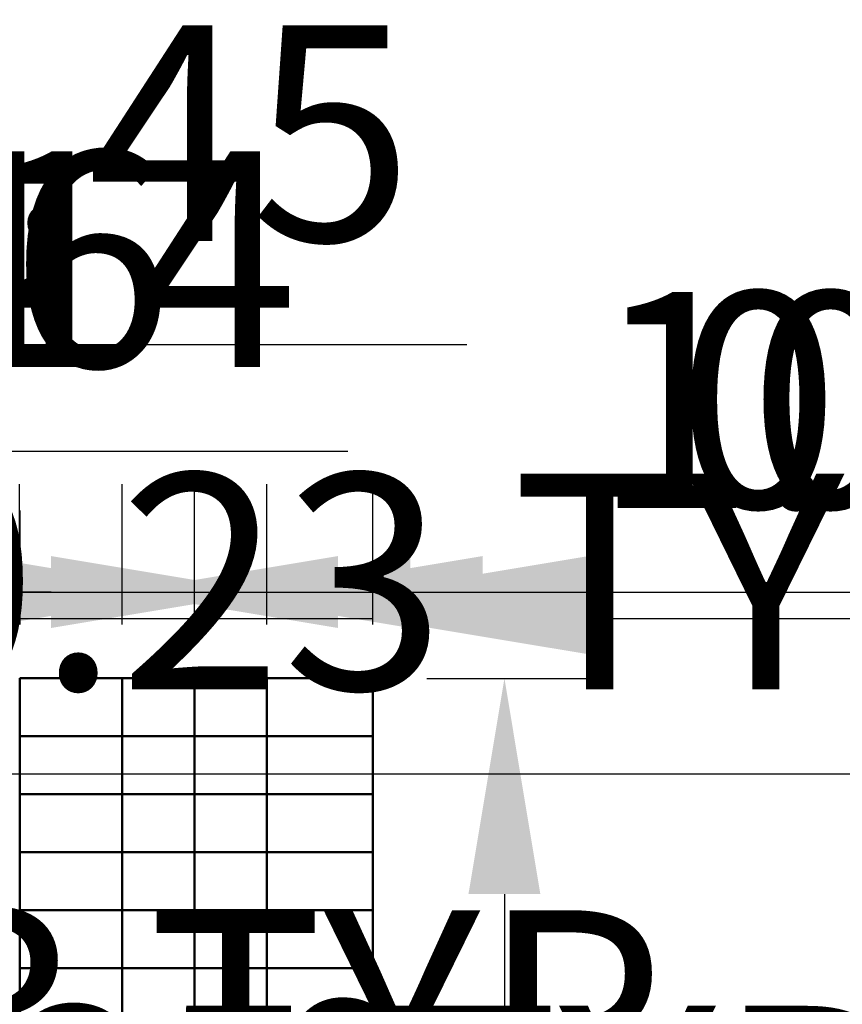
# Model space of a CAD drawing. Units: metres. Extents: x 782 to 1487, y 1262 to 7446.
# Tile 18 of 25: x 840.09 to 849.63, y 1302.06 to 1313.47. Entities that reach past the tile are written whole.
import ezdxf

# ---------------------------------------------------------------- set-up
doc = ezdxf.new("R2010")
doc.units = ezdxf.units.M
doc.layers.add('A-ANNO-DIMS', color=2, linetype='Continuous', lineweight=18)
doc.layers.add('A-WALL', color=7, linetype='Continuous', lineweight=50)
doc.styles.get("Standard").update_dxf_attribs({"font": 'arial.ttf'})
doc.dimstyles.new('ISO-25', dxfattribs={"dimtxt": 2.5, "dimasz": 2.5, "dimexe": 1.25, "dimexo": 0.625, "dimtad": 1, "dimtxsty": 'Standard', "dimcen": 2.5, "dimadec": 0, "dimazin": 0, "dimtfac": 1, "dimtmove": 0, "dimatfit": 3, "dimfxl": 1, "dimarcsym": 0})

# ---------------------------------------------------------------- blocks, each defined once
blk = doc.blocks.new('*D7')
at = {"layer": 'A-ANNO-DIMS', "color": 0, "lineweight": -2, "transparency": 16777216}
for p, q in [((827.962, 1307.952), (827.962, 1310.955)), ((832.412, 1307.952), (832.412, 1310.955)), ((825.462, 1309.705), (822.962, 1309.705)), ((827.962, 1309.705), (832.412, 1309.705)), ((834.912, 1309.705), (845.276, 1309.705))]:
    blk.add_line(p, q, dxfattribs=at)
at = {"layer": 'A-ANNO-DIMS', "color": 0, "transparency": 16777216}
for points in [[(825.462, 1310.122), (825.462, 1309.289), (827.962, 1309.705)], [(834.912, 1310.122), (834.912, 1309.289), (832.412, 1309.705)]]:
    blk.add_solid(points, dxfattribs=at)
at = {"layer": 'Defpoints', "color": 0, "transparency": 16777216}
for p in [(832.412, 1309.705), (827.962, 1307.327), (832.412, 1307.327)]:
    blk.add_point(p, dxfattribs=at)
at = {"layer": 'A-ANNO-DIMS', "color": 0, "transparency": 16777216, "insert": (841.344, 1311.828), "char_height": 2.5, "attachment_point": 5}
blk.add_mtext('4,45', dxfattribs=at)
blk = doc.blocks.new('*D8')
at = {"layer": 'A-ANNO-DIMS', "color": 0, "lineweight": -2, "transparency": 16777216}
for p, q in [((844.81, 1305.835), (846.96, 1305.835)), ((845.71, 1303.335), (845.71, 1292.805)), ((844.81, 1290.305), (846.96, 1290.305))]:
    blk.add_line(p, q, dxfattribs=at)
at = {"layer": 'A-ANNO-DIMS', "color": 0, "transparency": 16777216}
for points in [[(845.293, 1303.335), (846.126, 1303.335), (845.71, 1305.835)], [(845.293, 1292.805), (846.126, 1292.805), (845.71, 1290.305)]]:
    blk.add_solid(points, dxfattribs=at)
at = {"layer": 'Defpoints', "color": 0, "transparency": 16777216}
for p in [(844.185, 1305.835), (844.185, 1290.305), (845.71, 1290.305)]:
    blk.add_point(p, dxfattribs=at)
at = {"layer": 'A-ANNO-DIMS', "color": 0, "transparency": 16777216, "insert": (843.582, 1298.07), "char_height": 2.5, "attachment_point": 5, "rotation": 90}
blk.add_mtext('15,53', dxfattribs=at)
blk = doc.blocks.new('*D9')
at = {"layer": 'A-ANNO-DIMS', "color": 0, "lineweight": -2, "transparency": 16777216}
for p, q in [((840.095, 1306.46), (840.095, 1307.78)), ((844.185, 1306.46), (844.185, 1307.78)), ((837.595, 1306.53), (835.095, 1306.53)), ((840.095, 1306.53), (844.185, 1306.53)), ((846.685, 1306.53), (857.034, 1306.53))]:
    blk.add_line(p, q, dxfattribs=at)
at = {"layer": 'A-ANNO-DIMS', "color": 0, "transparency": 16777216}
for points in [[(837.595, 1306.947), (837.595, 1306.114), (840.095, 1306.53)], [(846.685, 1306.947), (846.685, 1306.114), (844.185, 1306.53)]]:
    blk.add_solid(points, dxfattribs=at)
at = {"layer": 'Defpoints', "color": 0, "transparency": 16777216}
for p in [(844.185, 1306.53), (840.095, 1305.835), (844.185, 1305.835)]:
    blk.add_point(p, dxfattribs=at)
at = {"layer": 'A-ANNO-DIMS', "color": 0, "transparency": 16777216, "insert": (853.11, 1308.658), "char_height": 2.5, "attachment_point": 5}
blk.add_mtext('4,09', dxfattribs=at)
blk = doc.blocks.new('*D21')
at = {"layer": 'A-ANNO-DIMS', "color": 0, "lineweight": -2, "transparency": 16777216}
for p, q in [((827.576, 1298.565), (825.076, 1298.565)), ((830.076, 1298.565), (830.923, 1298.565)), ((833.423, 1298.565), (852.255, 1298.565)), ((830.076, 1298.073), (830.076, 1297.315)), ((830.923, 1298.073), (830.923, 1297.315))]:
    blk.add_line(p, q, dxfattribs=at)
at = {"layer": 'A-ANNO-DIMS', "color": 0, "transparency": 16777216}
for points in [[(827.576, 1298.981), (827.576, 1298.148), (830.076, 1298.565)], [(833.423, 1298.981), (833.423, 1298.148), (830.923, 1298.565)]]:
    blk.add_solid(points, dxfattribs=at)
at = {"layer": 'Defpoints', "color": 0, "transparency": 16777216}
for p in [(830.076, 1298.698), (830.923, 1298.698), (830.923, 1298.565)]:
    blk.add_point(p, dxfattribs=at)
at = {"layer": 'A-ANNO-DIMS', "color": 0, "transparency": 16777216, "insert": (844.089, 1300.466), "char_height": 2.5, "attachment_point": 5}
blk.add_mtext('0.85 TYP.', dxfattribs=at)
blk = doc.blocks.new('*D24')
at = {"layer": 'A-ANNO-DIMS', "color": 0, "lineweight": -2, "transparency": 16777216}
for p, q in [((811.209, 1294.423), (808.709, 1294.423)), ((813.709, 1294.423), (814.559, 1294.423)), ((817.059, 1294.423), (852.649, 1294.423)), ((813.709, 1293.926), (813.709, 1293.173)), ((814.559, 1293.926), (814.559, 1293.173))]:
    blk.add_line(p, q, dxfattribs=at)
at = {"layer": 'A-ANNO-DIMS', "color": 0, "transparency": 16777216}
for points in [[(811.209, 1294.84), (811.209, 1294.006), (813.709, 1294.423)], [(817.059, 1294.84), (817.059, 1294.006), (814.559, 1294.423)]]:
    blk.add_solid(points, dxfattribs=at)
at = {"layer": 'Defpoints', "color": 0, "transparency": 16777216}
for p in [(813.709, 1294.551), (814.559, 1294.551), (814.559, 1294.423)]:
    blk.add_point(p, dxfattribs=at)
at = {"layer": 'A-ANNO-DIMS', "color": 0, "transparency": 16777216, "insert": (836.104, 1296.342), "char_height": 2.5, "attachment_point": 5}
blk.add_mtext('DOOR D2 0.85 TYP.', dxfattribs=at)
blk = doc.blocks.new('*D27')
at = {"layer": 'A-ANNO-DIMS', "color": 0, "lineweight": -2, "transparency": 16777216}
for p, q in [((825.463, 1299.672), (822.963, 1299.672)), ((827.963, 1299.672), (828.193, 1299.672)), ((830.693, 1299.672), (849.525, 1299.672)), ((827.963, 1299.184), (827.963, 1298.422)), ((828.193, 1299.184), (828.193, 1298.422))]:
    blk.add_line(p, q, dxfattribs=at)
at = {"layer": 'A-ANNO-DIMS', "color": 0, "transparency": 16777216}
for points in [[(825.463, 1300.088), (825.463, 1299.255), (827.963, 1299.672)], [(830.693, 1300.088), (830.693, 1299.255), (828.193, 1299.672)]]:
    blk.add_solid(points, dxfattribs=at)
at = {"layer": 'Defpoints', "color": 0, "transparency": 16777216}
for p in [(827.963, 1299.809), (828.193, 1299.809), (828.193, 1299.672)]:
    blk.add_point(p, dxfattribs=at)
at = {"layer": 'A-ANNO-DIMS', "color": 0, "transparency": 16777216, "insert": (841.359, 1301.574), "char_height": 2.5, "attachment_point": 5}
blk.add_mtext('0.23 TYP.', dxfattribs=at)
blk = doc.blocks.new('*D29')
at = {"layer": 'A-ANNO-DIMS', "color": 0, "lineweight": -2, "transparency": 16777216}
for p, q in [((829.683, 1304.73), (827.183, 1304.73)), ((832.183, 1304.73), (832.413, 1304.73)), ((834.913, 1304.73), (853.745, 1304.73)), ((832.183, 1304.242), (832.183, 1303.48)), ((832.413, 1304.242), (832.413, 1303.48))]:
    blk.add_line(p, q, dxfattribs=at)
at = {"layer": 'A-ANNO-DIMS', "color": 0, "transparency": 16777216}
for points in [[(829.683, 1305.146), (829.683, 1304.313), (832.183, 1304.73)], [(834.913, 1305.146), (834.913, 1304.313), (832.413, 1304.73)]]:
    blk.add_solid(points, dxfattribs=at)
at = {"layer": 'Defpoints', "color": 0, "transparency": 16777216}
for p in [(832.183, 1304.867), (832.413, 1304.867), (832.413, 1304.73)]:
    blk.add_point(p, dxfattribs=at)
at = {"layer": 'A-ANNO-DIMS', "color": 0, "transparency": 16777216, "insert": (845.579, 1306.632), "char_height": 2.5, "attachment_point": 5}
blk.add_mtext('0.23 TYP.', dxfattribs=at)
blk = doc.blocks.new('*D94')
at = {"layer": 'A-ANNO-DIMS', "color": 0, "lineweight": -2, "transparency": 16777216}
for p, q in [((827.962, 1307.952), (827.962, 1309.718)), ((828.406, 1307.953), (828.406, 1309.718)), ((825.462, 1308.468), (822.962, 1308.468)), ((827.962, 1308.468), (828.406, 1308.468)), ((830.906, 1308.468), (841.139, 1308.468))]:
    blk.add_line(p, q, dxfattribs=at)
at = {"layer": 'A-ANNO-DIMS', "color": 0, "transparency": 16777216}
for points in [[(825.462, 1308.884), (825.462, 1308.051), (827.962, 1308.468)], [(830.906, 1308.884), (830.906, 1308.051), (828.406, 1308.468)]]:
    blk.add_solid(points, dxfattribs=at)
at = {"layer": 'Defpoints', "color": 0, "transparency": 16777216}
for p in [(828.406, 1308.468), (827.962, 1307.327), (828.406, 1307.328)]:
    blk.add_point(p, dxfattribs=at)
at = {"layer": 'A-ANNO-DIMS', "color": 0, "transparency": 16777216, "insert": (837.273, 1310.369), "char_height": 2.5, "attachment_point": 5}
blk.add_mtext('0.44', dxfattribs=at)
blk = doc.blocks.new('*D95')
at = {"layer": 'A-ANNO-DIMS', "color": 0, "lineweight": -2, "transparency": 16777216}
for p, q in [((828.406, 1307.953), (828.406, 1309.718)), ((829.22, 1307.953), (829.22, 1309.718)), ((825.906, 1308.468), (823.406, 1308.468)), ((828.406, 1308.468), (829.22, 1308.468)), ((831.72, 1308.468), (843.896, 1308.468))]:
    blk.add_line(p, q, dxfattribs=at)
at = {"layer": 'A-ANNO-DIMS', "color": 0, "transparency": 16777216}
for points in [[(825.906, 1308.884), (825.906, 1308.051), (828.406, 1308.468)], [(831.72, 1308.884), (831.72, 1308.051), (829.22, 1308.468)]]:
    blk.add_solid(points, dxfattribs=at)
at = {"layer": 'Defpoints', "color": 0, "transparency": 16777216}
for p in [(829.22, 1308.468), (828.406, 1307.328), (829.22, 1307.328)]:
    blk.add_point(p, dxfattribs=at)
at = {"layer": 'A-ANNO-DIMS', "color": 0, "transparency": 16777216, "insert": (839.058, 1310.369), "char_height": 2.5, "attachment_point": 5}
blk.add_mtext('0.814', dxfattribs=at)
blk = doc.blocks.new('*D96')
at = {"layer": 'A-ANNO-DIMS', "color": 0, "lineweight": -2, "transparency": 16777216}
for p, q in [((829.22, 1307.953), (829.22, 1309.718)), ((829.682, 1307.722), (829.682, 1309.718)), ((826.72, 1308.468), (824.22, 1308.468)), ((829.22, 1308.468), (829.682, 1308.468)), ((832.182, 1308.468), (842.425, 1308.468))]:
    blk.add_line(p, q, dxfattribs=at)
at = {"layer": 'A-ANNO-DIMS', "color": 0, "transparency": 16777216}
for points in [[(826.72, 1308.884), (826.72, 1308.051), (829.22, 1308.468)], [(832.182, 1308.884), (832.182, 1308.051), (829.682, 1308.468)]]:
    blk.add_solid(points, dxfattribs=at)
at = {"layer": 'Defpoints', "color": 0, "transparency": 16777216}
for p in [(829.682, 1308.468), (829.22, 1307.328), (829.682, 1307.097)]:
    blk.add_point(p, dxfattribs=at)
at = {"layer": 'A-ANNO-DIMS', "color": 0, "transparency": 16777216, "insert": (838.554, 1310.369), "char_height": 2.5, "attachment_point": 5}
blk.add_mtext('0.46', dxfattribs=at)
blk = doc.blocks.new('*D101')
at = {"layer": 'A-ANNO-DIMS', "color": 0, "lineweight": -2, "transparency": 16777216}
for p, q in [((840.091, 1306.46), (840.091, 1308.085)), ((841.28, 1306.46), (841.28, 1308.085)), ((837.591, 1306.835), (835.091, 1306.835)), ((840.091, 1306.835), (841.28, 1306.835)), ((843.78, 1306.835), (853.794, 1306.835))]:
    blk.add_line(p, q, dxfattribs=at)
at = {"layer": 'A-ANNO-DIMS', "color": 0, "transparency": 16777216}
for points in [[(837.591, 1307.252), (837.591, 1306.419), (840.091, 1306.835)], [(843.78, 1307.252), (843.78, 1306.419), (841.28, 1306.835)]]:
    blk.add_solid(points, dxfattribs=at)
at = {"layer": 'Defpoints', "color": 0, "transparency": 16777216}
for p in [(841.28, 1306.835), (840.091, 1305.835), (841.28, 1305.835)]:
    blk.add_point(p, dxfattribs=at)
at = {"layer": 'A-ANNO-DIMS', "color": 0, "transparency": 16777216, "insert": (850.037, 1308.737), "char_height": 2.5, "attachment_point": 5}
blk.add_mtext('1.19', dxfattribs=at)
blk = doc.blocks.new('*D102')
at = {"layer": 'A-ANNO-DIMS', "color": 0, "lineweight": -2, "transparency": 16777216}
for p, q in [((841.28, 1306.46), (841.28, 1308.085)), ((842.118, 1306.46), (842.118, 1308.085)), ((838.78, 1306.835), (836.28, 1306.835)), ((841.28, 1306.835), (842.118, 1306.835)), ((844.618, 1306.835), (856.81, 1306.835))]:
    blk.add_line(p, q, dxfattribs=at)
at = {"layer": 'A-ANNO-DIMS', "color": 0, "transparency": 16777216}
for points in [[(838.78, 1307.252), (838.78, 1306.419), (841.28, 1306.835)], [(844.618, 1307.252), (844.618, 1306.419), (842.118, 1306.835)]]:
    blk.add_solid(points, dxfattribs=at)
at = {"layer": 'Defpoints', "color": 0, "transparency": 16777216}
for p in [(842.118, 1306.835), (841.28, 1305.835), (842.118, 1305.835)]:
    blk.add_point(p, dxfattribs=at)
at = {"layer": 'A-ANNO-DIMS', "color": 0, "transparency": 16777216, "insert": (851.964, 1308.738), "char_height": 2.5, "attachment_point": 5}
blk.add_mtext('0.838', dxfattribs=at)
blk = doc.blocks.new('*D103')
at = {"layer": 'A-ANNO-DIMS', "color": 0, "lineweight": -2, "transparency": 16777216}
for p, q in [((842.118, 1306.46), (842.118, 1308.085)), ((842.956, 1306.46), (842.956, 1308.085)), ((839.618, 1306.835), (837.118, 1306.835)), ((842.118, 1306.835), (842.956, 1306.835)), ((845.456, 1306.835), (857.648, 1306.835))]:
    blk.add_line(p, q, dxfattribs=at)
at = {"layer": 'A-ANNO-DIMS', "color": 0, "transparency": 16777216}
for points in [[(839.618, 1307.252), (839.618, 1306.419), (842.118, 1306.835)], [(845.456, 1307.252), (845.456, 1306.419), (842.956, 1306.835)]]:
    blk.add_solid(points, dxfattribs=at)
at = {"layer": 'Defpoints', "color": 0, "transparency": 16777216}
for p in [(842.956, 1306.835), (842.118, 1305.835), (842.956, 1305.835)]:
    blk.add_point(p, dxfattribs=at)
at = {"layer": 'A-ANNO-DIMS', "color": 0, "transparency": 16777216, "insert": (852.802, 1308.738), "char_height": 2.5, "attachment_point": 5}
blk.add_mtext('0.838', dxfattribs=at)
blk = doc.blocks.new('*D104')
at = {"layer": 'A-ANNO-DIMS', "color": 0, "lineweight": -2, "transparency": 16777216}
for p, q in [((842.956, 1306.46), (842.956, 1308.085)), ((844.185, 1306.46), (844.185, 1308.085)), ((840.456, 1306.835), (837.956, 1306.835)), ((842.956, 1306.835), (844.185, 1306.835)), ((846.685, 1306.835), (856.693, 1306.835))]:
    blk.add_line(p, q, dxfattribs=at)
at = {"layer": 'A-ANNO-DIMS', "color": 0, "transparency": 16777216}
for points in [[(840.456, 1307.252), (840.456, 1306.419), (842.956, 1306.835)], [(846.685, 1307.252), (846.685, 1306.419), (844.185, 1306.835)]]:
    blk.add_solid(points, dxfattribs=at)
at = {"layer": 'Defpoints', "color": 0, "transparency": 16777216}
for p in [(844.185, 1306.835), (842.956, 1305.835), (844.185, 1305.835)]:
    blk.add_point(p, dxfattribs=at)
at = {"layer": 'A-ANNO-DIMS', "color": 0, "transparency": 16777216, "insert": (852.939, 1308.738), "char_height": 2.5, "attachment_point": 5}
blk.add_mtext('1.23', dxfattribs=at)

msp = doc.modelspace()

# ---------------------------------------------------------------- linework, layer by layer
at = {"layer": 'A-WALL'}
for p, q in [((840.0913, 1305.8353), (844.1849, 1305.8353)), ((844.1849, 1305.8353), (840.0949, 1305.8353)), ((840.0949, 1305.8353), (840.0949, 1290.3053)), ((841.2801, 1305.8353), (842.9563, 1305.8353)), ((841.2801, 1300.4593), (841.2801, 1305.8353)), ((842.1182, 1305.8353), (842.1182, 1300.4593)), ((842.9563, 1305.8353), (842.9563, 1300.4593)), ((844.1849, 1290.3053), (844.1849, 1305.8353)), ((840.0913, 1305.1633), (844.1849, 1305.1633)), ((840.0913, 1304.4913), (844.1849, 1304.4913)), ((840.0913, 1303.8193), (844.1849, 1303.8193)), ((840.0913, 1303.1473), (844.1849, 1303.1473)), ((840.0913, 1302.4753), (844.1849, 1302.4753))]:
    msp.add_line(p, q, dxfattribs=at)

# ---------------------------------------------------------------- dimensions: what is measured, and where the dimension line sits
at = {"layer": 'A-ANNO-DIMS'}
for base, p1, p2, override, picture, middle in [((832.4125, 1309.7054), (827.9625, 1307.3274), (832.4125, 1307.3274), {"dimclrd": 0, "dimclre": 0, "dimclrt": 0}, '*D7', (841.3441, 1311.8277)), ((828.4057, 1308.4676), (827.9625, 1307.3274), (828.4057, 1307.3276), {"dimdec": 2, "dimlfac": 1, "dimrnd": 0, "dimzin": 0, "dimdsep": 46, "dimlunit": 2}, '*D94', (837.2725, 1310.369)), ((829.2197, 1308.4676), (828.4057, 1307.3276), (829.2197, 1307.3276), {"dimdec": 3, "dimlfac": 1, "dimrnd": 0, "dimzin": 0, "dimdsep": 46, "dimlunit": 2}, '*D95', (839.0577, 1310.369)), ((829.6825, 1308.4676), (829.2197, 1307.3276), (829.6825, 1307.0974), {"dimdec": 2, "dimlfac": 1, "dimrnd": 0, "dimzin": 0, "dimdsep": 46, "dimlunit": 2}, '*D96', (838.5536, 1310.369)), ((841.2801, 1306.8353), (840.0913, 1305.8353), (841.2801, 1305.8353), {"dimdec": 2, "dimlfac": 1, "dimrnd": 0, "dimzin": 0, "dimdsep": 46, "dimlunit": 2}, '*D101', (850.037, 1308.7367)), ((844.1849, 1306.5303), (840.0949, 1305.8353), (844.1849, 1305.8353), {"dimclrd": 0, "dimclre": 0, "dimclrt": 0}, '*D9', (853.1097, 1308.6577)), ((842.1182, 1306.8353), (841.2801, 1305.8353), (842.1182, 1305.8353), {"dimdec": 3, "dimlfac": 1, "dimrnd": 0, "dimzin": 0, "dimdsep": 46, "dimlunit": 2}, '*D102', (851.9639, 1308.7376)), ((842.9563, 1306.8353), (842.1182, 1305.8353), (842.9563, 1305.8353), {"dimdec": 3, "dimlfac": 1, "dimrnd": 0, "dimzin": 0, "dimdsep": 46, "dimlunit": 2}, '*D103', (852.802, 1308.7376)), ((844.1849, 1306.8353), (842.9563, 1305.8353), (844.1849, 1305.8353), {"dimdec": 2, "dimlfac": 1, "dimrnd": 0, "dimzin": 0, "dimdsep": 46, "dimlunit": 2}, '*D104', (852.9391, 1308.7376))]:
    dim = msp.add_linear_dim(base=base, p1=p1, p2=p2, dimstyle='ISO-25', override=override, dxfattribs=at)
    dim.commit()
    dim.dimension.update_dxf_attribs({"geometry": picture, "text_midpoint": middle})
for base, p1, p2, text, picture, middle in [((832.4132, 1304.7298), (832.1832, 1304.8669), (832.4132, 1304.8669), '<> TYP.', '*D29', (845.5791, 1306.6321)), ((828.1931, 1299.6717), (827.9631, 1299.8088), (828.1931, 1299.8088), '<> TYP.', '*D27', (841.359, 1301.574)), ((814.5592, 1294.4231), (813.7086, 1294.5507), (814.5592, 1294.5507), 'DOOR D2 <> TYP.', '*D24', (836.1042, 1296.3416)), ((830.923, 1298.5648), (830.0763, 1298.6982), (830.923, 1298.6982), '<> TYP.', '*D21', (844.0889, 1300.4662))]:
    dim = msp.add_linear_dim(base=base, p1=p1, p2=p2, text=text, dimstyle='ISO-25', override={"dimdec": 2, "dimlfac": 1, "dimrnd": 0, "dimzin": 0, "dimdsep": 46, "dimlunit": 2}, dxfattribs=at)
    dim.commit()
    dim.dimension.update_dxf_attribs({"geometry": picture, "text_midpoint": middle})
dim = msp.add_linear_dim(base=(845.7096, 1290.3053), p1=(844.1849, 1305.8353), p2=(844.1849, 1290.3053), angle=90, dimstyle='ISO-25', override={"dimclrd": 0, "dimclre": 0, "dimclrt": 0}, dxfattribs=at)
dim.commit()
dim.dimension.update_dxf_attribs({"geometry": '*D8', "text_midpoint": (843.5822, 1298.0703)})

doc.saveas('drawing.dxf')
